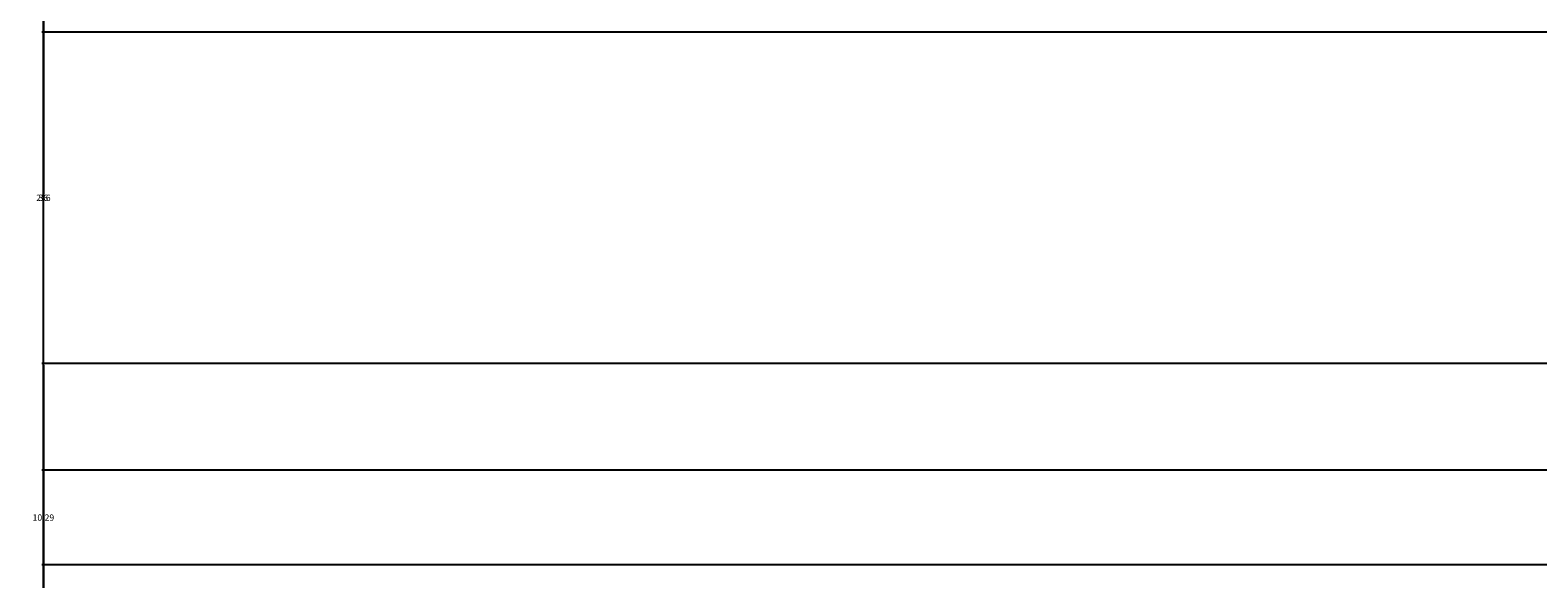
# Model space of a CAD drawing. Units: inches. Extents: x -145 to 510, y 5 to 386.
# Tile 7 of 25: x -145 to 18, y 177 to 236. Entities that reach past the tile are written whole.
import ezdxf

# ---------------------------------------------------------------- set-up
doc = ezdxf.new("R2010")
doc.units = ezdxf.units.IN
doc.header["$MEASUREMENT"] = 0
doc.layers.add('A-ANNO-DIMS', color=2, linetype='Continuous', lineweight=18)
doc.styles.get("Standard").update_dxf_attribs({"font": 'arial.ttf'})
doc.dimstyles.get("Standard").update_dxf_attribs({"dimtxt": 0.6875, "dimasz": 0.18, "dimexe": 0.18, "dimexo": 0.0625, "dimgap": 0.09, "dimtad": 0, "dimtih": 1, "dimtoh": 1, "dimdec": 4, "dimzin": 0, "dimdsep": 46, "dimlunit": 4, "dimtxsty": 'Standard', "dimcen": 0.09, "dimadec": 0, "dimazin": 0, "dimtfac": 1, "dimtdec": 4, "dimtofl": 0, "dimtmove": 0, "dimatfit": 3, "dimfxl": 1, "dimtolj": 1, "dimtzin": 0, "dimarcsym": 0})

# ---------------------------------------------------------------- blocks, each defined once
blk = doc.blocks.new('*D19')
at = {"layer": 'A-ANNO-DIMS', "color": 0, "lineweight": -2, "transparency": 16777216}
for p, q in [((478.76, 355.89), (-144.05, 355.89)), ((-143.87, 355.71), (-143.87, 218.33)), ((-143.87, 80.07), (-143.87, 217.45)), ((-114.04, 79.89), (-144.05, 79.89))]:
    blk.add_line(p, q, dxfattribs=at)
at = {"layer": 'A-ANNO-DIMS', "color": 0, "transparency": 16777216}
for points in [[(-143.9, 355.71), (-143.84, 355.71), (-143.87, 355.89)], [(-143.9, 80.07), (-143.84, 80.07), (-143.87, 79.89)]]:
    blk.add_solid(points, dxfattribs=at)
at = {"layer": 'Defpoints', "color": 0, "transparency": 16777216}
for p in [(-143.87, 355.89), (478.83, 355.89), (-113.97, 79.89)]:
    blk.add_point(p, dxfattribs=at)
at = {"layer": 'A-ANNO-DIMS', "color": 0, "transparency": 16777216, "insert": (-143.87, 217.89), "char_height": 0.688, "attachment_point": 5}
blk.add_mtext('\\A1;276', dxfattribs=at)
blk = doc.blocks.new('*D20')
at = {"layer": 'A-ANNO-DIMS', "color": 0, "lineweight": -2, "transparency": 16777216}
for p, q in [((53.94, 199.89), (-144.05, 199.89)), ((-143.87, 199.71), (-143.87, 140.33)), ((-143.87, 80.07), (-143.87, 139.45)), ((53.94, 79.89), (-144.05, 79.89))]:
    blk.add_line(p, q, dxfattribs=at)
at = {"layer": 'A-ANNO-DIMS', "color": 0, "transparency": 16777216}
for points in [[(-143.9, 199.71), (-143.84, 199.71), (-143.87, 199.89)], [(-143.9, 80.07), (-143.84, 80.07), (-143.87, 79.89)]]:
    blk.add_solid(points, dxfattribs=at)
at = {"layer": 'Defpoints', "color": 0, "transparency": 16777216}
for p in [(-143.87, 199.89), (54, 199.89), (54, 79.89)]:
    blk.add_point(p, dxfattribs=at)
at = {"layer": 'A-ANNO-DIMS', "color": 0, "transparency": 16777216, "insert": (-143.87, 139.89), "char_height": 0.688, "attachment_point": 5}
blk.add_mtext('\\A1;120', dxfattribs=at)
blk = doc.blocks.new('*D21')
at = {"layer": 'A-ANNO-DIMS', "color": 0, "lineweight": -2, "transparency": 16777216}
for p, q in [((34.21, 327.61), (-144.05, 327.61)), ((-143.87, 327.43), (-143.87, 264.19)), ((-143.87, 200.07), (-143.87, 263.31)), ((69.71, 199.89), (-144.05, 199.89))]:
    blk.add_line(p, q, dxfattribs=at)
at = {"layer": 'A-ANNO-DIMS', "color": 0, "transparency": 16777216}
for points in [[(-143.9, 327.43), (-143.84, 327.43), (-143.87, 327.61)], [(-143.9, 200.07), (-143.84, 200.07), (-143.87, 199.89)]]:
    blk.add_solid(points, dxfattribs=at)
at = {"layer": 'Defpoints', "color": 0, "transparency": 16777216}
for p in [(-143.87, 327.61), (34.27, 327.61), (69.78, 199.89)]:
    blk.add_point(p, dxfattribs=at)
at = {"layer": 'A-ANNO-DIMS', "color": 0, "transparency": 16777216, "insert": (-143.87, 263.75), "char_height": 0.688, "attachment_point": 5}
blk.add_mtext('\\A1;127.72', dxfattribs=at)
blk = doc.blocks.new('*D25')
at = {"layer": 'A-ANNO-DIMS', "color": 0, "lineweight": -2, "transparency": 16777216}
for p, q in [((74.44, 235.89), (-144.05, 235.89)), ((-143.87, 235.71), (-143.87, 218.33)), ((-143.87, 200.07), (-143.87, 217.45)), ((74.44, 199.89), (-144.05, 199.89))]:
    blk.add_line(p, q, dxfattribs=at)
at = {"layer": 'A-ANNO-DIMS', "color": 0, "transparency": 16777216}
for points in [[(-143.9, 235.71), (-143.84, 235.71), (-143.87, 235.89)], [(-143.9, 200.07), (-143.84, 200.07), (-143.87, 199.89)]]:
    blk.add_solid(points, dxfattribs=at)
at = {"layer": 'Defpoints', "color": 0, "transparency": 16777216}
for p in [(-143.87, 235.89), (74.51, 235.89), (74.51, 199.89)]:
    blk.add_point(p, dxfattribs=at)
at = {"layer": 'A-ANNO-DIMS', "color": 0, "transparency": 16777216, "insert": (-143.87, 217.89), "char_height": 0.688, "attachment_point": 5}
blk.add_mtext('\\A1;36', dxfattribs=at)
blk = doc.blocks.new('*D26')
at = {"layer": 'A-ANNO-DIMS', "color": 0, "lineweight": -2, "transparency": 16777216}
for p, q in [((95.08, 305.74), (-144.05, 305.74)), ((-143.87, 305.56), (-143.87, 253.26)), ((-143.87, 200.07), (-143.87, 252.38)), ((95.08, 199.89), (-144.05, 199.89))]:
    blk.add_line(p, q, dxfattribs=at)
at = {"layer": 'A-ANNO-DIMS', "color": 0, "transparency": 16777216}
for points in [[(-143.9, 305.56), (-143.84, 305.56), (-143.87, 305.74)], [(-143.9, 200.07), (-143.84, 200.07), (-143.87, 199.89)]]:
    blk.add_solid(points, dxfattribs=at)
at = {"layer": 'Defpoints', "color": 0, "transparency": 16777216}
for p in [(-143.87, 305.74), (95.14, 305.74), (95.14, 199.89)]:
    blk.add_point(p, dxfattribs=at)
at = {"layer": 'A-ANNO-DIMS', "color": 0, "transparency": 16777216, "insert": (-143.87, 252.82), "char_height": 0.688, "attachment_point": 5}
blk.add_mtext('\\A1;105.85', dxfattribs=at)
blk = doc.blocks.new('*D27')
at = {"layer": 'A-ANNO-DIMS', "color": 0, "lineweight": -2, "transparency": 16777216}
for p, q in [((244.23, 279.84), (-144.05, 279.84)), ((-143.87, 279.66), (-143.87, 240.31)), ((-143.87, 200.07), (-143.87, 239.43)), ((218.29, 199.89), (-144.05, 199.89))]:
    blk.add_line(p, q, dxfattribs=at)
at = {"layer": 'A-ANNO-DIMS', "color": 0, "transparency": 16777216}
for points in [[(-143.9, 279.66), (-143.84, 279.66), (-143.87, 279.84)], [(-143.9, 200.07), (-143.84, 200.07), (-143.87, 199.89)]]:
    blk.add_solid(points, dxfattribs=at)
at = {"layer": 'Defpoints', "color": 0, "transparency": 16777216}
for p in [(-143.87, 279.84), (244.29, 279.84), (218.36, 199.89)]:
    blk.add_point(p, dxfattribs=at)
at = {"layer": 'A-ANNO-DIMS', "color": 0, "transparency": 16777216, "insert": (-143.87, 239.87), "char_height": 0.688, "attachment_point": 5}
blk.add_mtext('\\A1;79.95', dxfattribs=at)
blk = doc.blocks.new('*D30')
at = {"layer": 'A-ANNO-DIMS', "color": 0, "lineweight": -2, "transparency": 16777216}
for p, q in [((210.73, 188.31), (-144.05, 188.31)), ((-143.87, 188.13), (-143.87, 183.61)), ((-143.87, 178.2), (-143.87, 182.72)), ((210.73, 178.02), (-144.05, 178.02))]:
    blk.add_line(p, q, dxfattribs=at)
at = {"layer": 'A-ANNO-DIMS', "color": 0, "transparency": 16777216}
for points in [[(-143.9, 188.13), (-143.84, 188.13), (-143.87, 188.31)], [(-143.9, 178.2), (-143.84, 178.2), (-143.87, 178.02)]]:
    blk.add_solid(points, dxfattribs=at)
at = {"layer": 'Defpoints', "color": 0, "transparency": 16777216}
for p in [(-143.87, 188.31), (210.8, 188.31), (210.8, 178.02)]:
    blk.add_point(p, dxfattribs=at)
at = {"layer": 'A-ANNO-DIMS', "color": 0, "transparency": 16777216, "insert": (-143.87, 183.16), "char_height": 0.688, "attachment_point": 5}
blk.add_mtext('\\A1;10.29', dxfattribs=at)

msp = doc.modelspace()

# ---------------------------------------------------------------- dimensions: what is measured, and where the dimension line sits
at = {"layer": 'A-ANNO-DIMS'}
for base, p1, p2, override, picture, middle in [((-143.8737, 355.8905), (-113.9737, 79.8905), (478.8263, 355.8905), {"dimdec": 0, "dimlfac": 1, "dimrnd": 0, "dimzin": 0, "dimdsep": 46, "dimlunit": 2}, '*D19', (-143.8737, 217.8905)), ((-143.8737, 327.6093), (69.7763, 199.8905), (34.2706, 327.6093), {"dimdec": 2, "dimlfac": 1, "dimrnd": 0, "dimzin": 0, "dimdsep": 46, "dimlunit": 2}, '*D21', (-143.8737, 263.7499)), ((-143.8737, 305.7416), (95.1414, 199.8905), (95.1414, 305.7416), {"dimdec": 2, "dimlfac": 1, "dimrnd": 0, "dimzin": 0, "dimdsep": 46, "dimlunit": 2}, '*D26', (-143.8737, 252.8161)), ((-143.8737, 279.8443), (218.3571, 199.8905), (244.2916, 279.8443), {"dimdec": 2, "dimlfac": 1, "dimrnd": 0, "dimzin": 0, "dimdsep": 46, "dimlunit": 2}, '*D27', (-143.8737, 239.8674)), ((-143.8737, 235.8905), (74.5073, 199.8905), (74.5073, 235.8905), {"dimdec": 0, "dimlfac": 1, "dimrnd": 0, "dimzin": 0, "dimdsep": 46, "dimlunit": 2}, '*D25', (-143.8737, 217.8905)), ((-143.8737, 199.8905), (54.0014, 79.8905), (54.0014, 199.8905), {"dimdec": 0, "dimlfac": 1, "dimrnd": 0, "dimzin": 0, "dimdsep": 46, "dimlunit": 2}, '*D20', (-143.8737, 139.8905)), ((-143.8737, 188.3087), (210.7973, 178.0195), (210.7973, 188.3087), {"dimdec": 2, "dimlfac": 1, "dimrnd": 0, "dimzin": 0, "dimdsep": 46, "dimlunit": 2}, '*D30', (-143.8737, 183.1641))]:
    dim = msp.add_linear_dim(base=base, p1=p1, p2=p2, angle=90, dimstyle='Standard', override=override, dxfattribs=at)
    dim.commit()
    dim.dimension.update_dxf_attribs({"geometry": picture, "text_midpoint": middle})

doc.saveas('drawing.dxf')
